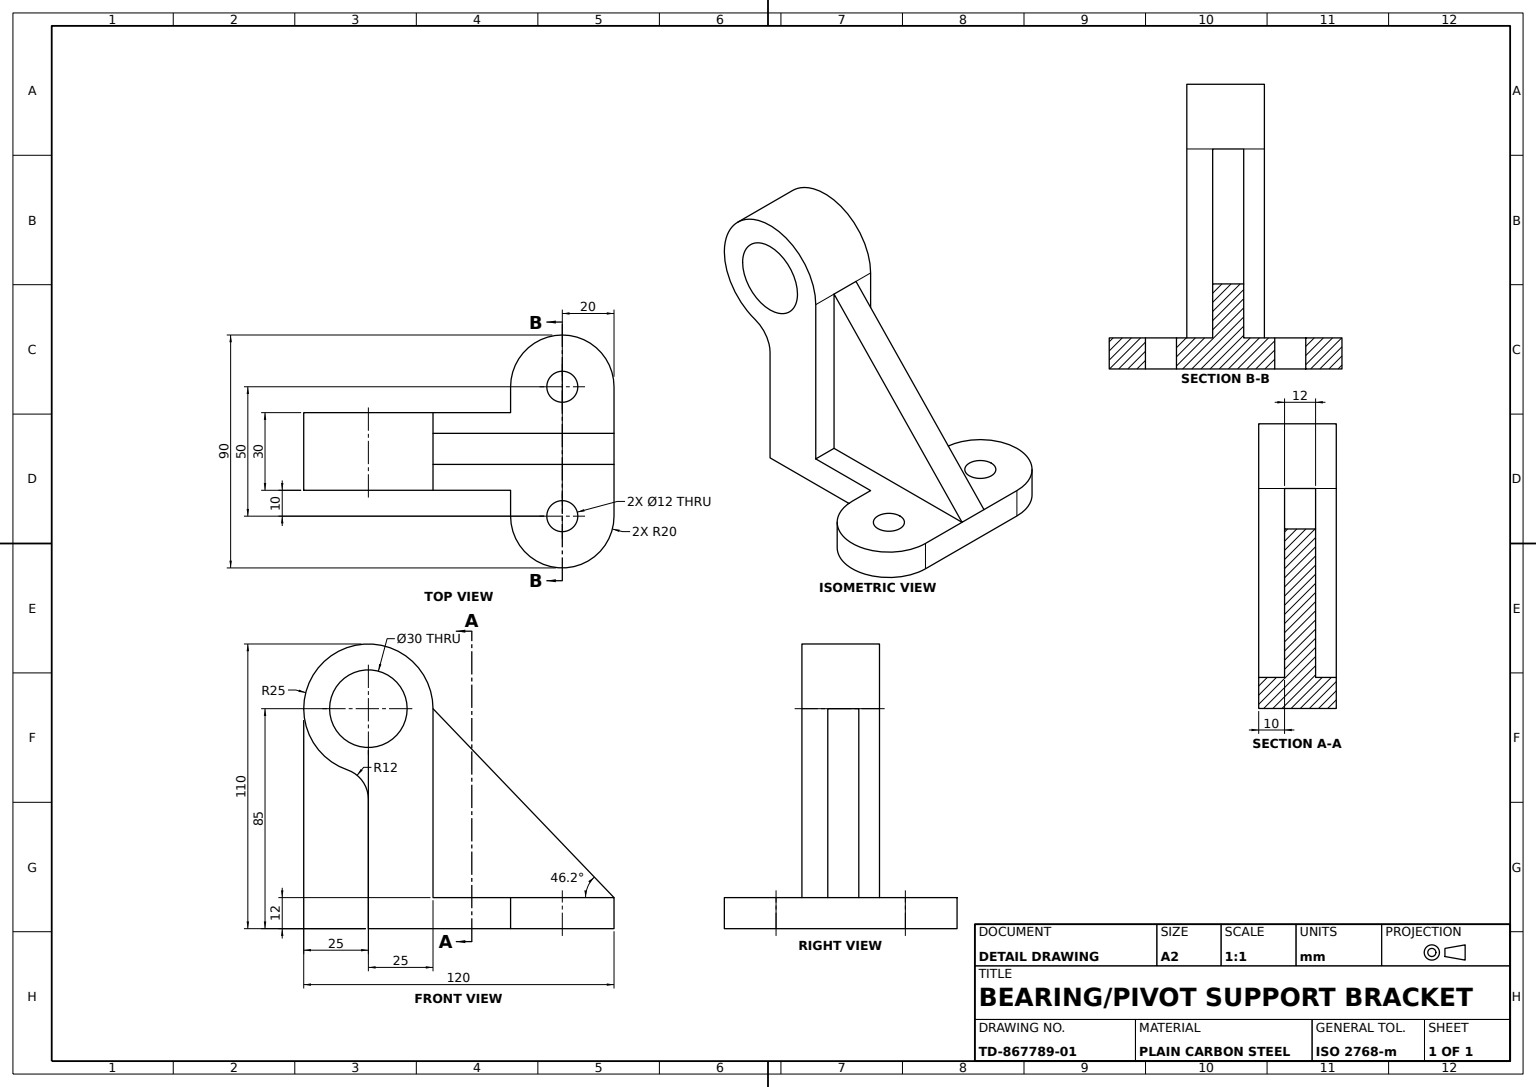
SolidWorks part; units mm, degrees
material "Plain Carbon Steel"
ref_plane "Front Plane" through (0, 0, 0) normal (0, 0, 1) x (1, 0, 0)
ref_plane "Top Plane" through (0, 0, 0) normal (0, 1, 0) x (1, 0, 0)
ref_plane "Right Plane" through (0, 0, 0) normal (1, 0, 0) x (0, 0, -1)
sketch "Base Plate Sketch" plane through (0, 0, 0) normal (0, 1, 0) x (1, 0, 0)
  line L0 (-74.684, 0) -> (63.7107, 0) construction
  line L1 (0, -25) -> (0, 37.8193) construction
  line L2 (-20, 25) -> (-20, 15)
  line L3 (-20, 15) -> (-50, 15)
  line L4 (-20, -25) -> (-20, -15)
  line L5 (-20, -15) -> (-50, -15)
  line L6 (-50, -15) -> (-50, 15)
  line L7 (20, 25) -> (20, -25)
  circle A0 centre (0, 25) radius 6
  arc A1 (20, 25) -> (-20, 25) centre (0, 25) ccw
  circle A2 centre (0, -25) radius 6
  arc A3 (-20, -25) -> (20, -25) centre (0, -25) ccw
  dimension "D1" = 40
  dimension "D2" = 12
  dimension "D3" = 12
  dimension "D4" = 50
  dimension "D5" = 15
  dimension "D6" = 50
  dimension "25" = 25
  dimension "30" = 30
extrude "Base Plate" add sketch "Base Plate Sketch" along normal mid plane 12
sketch "Upright Bore Sketch" plane through (0, 0, 0) normal (0, 0, 1) x (1, 0, 0)
  line L0 (-50, -6) -> (-75, -6)
  line L1 (-75, -6) -> (-75, 44)
  line L3 (-50, 79) -> (-50, -6)
  arc A0 (-50, 79) -> (-83.1081, 55.3514) centre (-75, 79) ccw
  circle A1 centre (-75, 79) radius 15
  arc A2 (-75, 44) -> (-83.1081, 55.3514) centre (-87, 44) ccw
  dimension "D3" = 30
  dimension "50" = 50
  dimension "D2" = 12
  dimension "D1" = 85
extrude "Upright with Bore" add sketch "Upright Bore Sketch" along normal mid plane 30
sketch "Rib Layout Sketch" plane through (0, 0, 0) normal (1, 0, 0) x (0, 0, -1)
  line L0 (-5, 6) -> (-5, 79)
  line L1 (15, 6) -> (-15, 6) construction
  line L2 (-15, 79) -> (15, 79) construction
  line L3 (-5, 79) -> (7, 79)
  line L4 (7, 79) -> (7, 6)
  line L5 (7, 6) -> (-5, 6)
  dimension "D1" = 12
  dimension "D2" = 5
sketch "Rib Sketch" plane through (-50, 0, 0) normal (1, 0, 0) x (0, 0, -1)
  line L0 (-5, 6) -> (-5, 79) construction
  line L1 (-5, 6) -> (-5, 79)
  line L2 (-5, 79) -> (7, 79) construction
  line L3 (-5, 79) -> (7, 79)
  line L4 (-15, 6) -> (15, 6)
  line L5 (15, 6) -> (15, 79)
  line L6 (15, 79) -> (-15, 79)
  line L7 (-15, 79) -> (-15, 6)
  line L8 (-15, 6) -> (15, 6)
  line L9 (15, 6) -> (15, 79)
  line L11 (-15, 79) -> (-15, 6)
  line L12 (7, 79) -> (7, 6) construction
  line L13 (7, 79) -> (7, 6)
  line L14 (7, 6) -> (-5, 6) construction
  line L15 (7, 6) -> (-5, 6)
  line M9 (-15, 6) -> (15, 6)
  line M11 (15, 79) -> (-15, 79)
  dimension "D1" = 0
extrude "Rib" add sketch "Rib Sketch" along normal blind 70 contours L13 L1 M11 M9
sketch "Rib Wedge Cut Sketch" plane through (0, 0, 5) normal (0, 0, 1) x (1, 0, 0)
  line L0 (20, 6) -> (-50, 79)
  line L1 (-50, 79) -> (20, 79)
  line L2 (20, 79) -> (20, 6)
extrude "Rib Wedge Cut" cut sketch "Rib Wedge Cut Sketch" against normal blind 70
